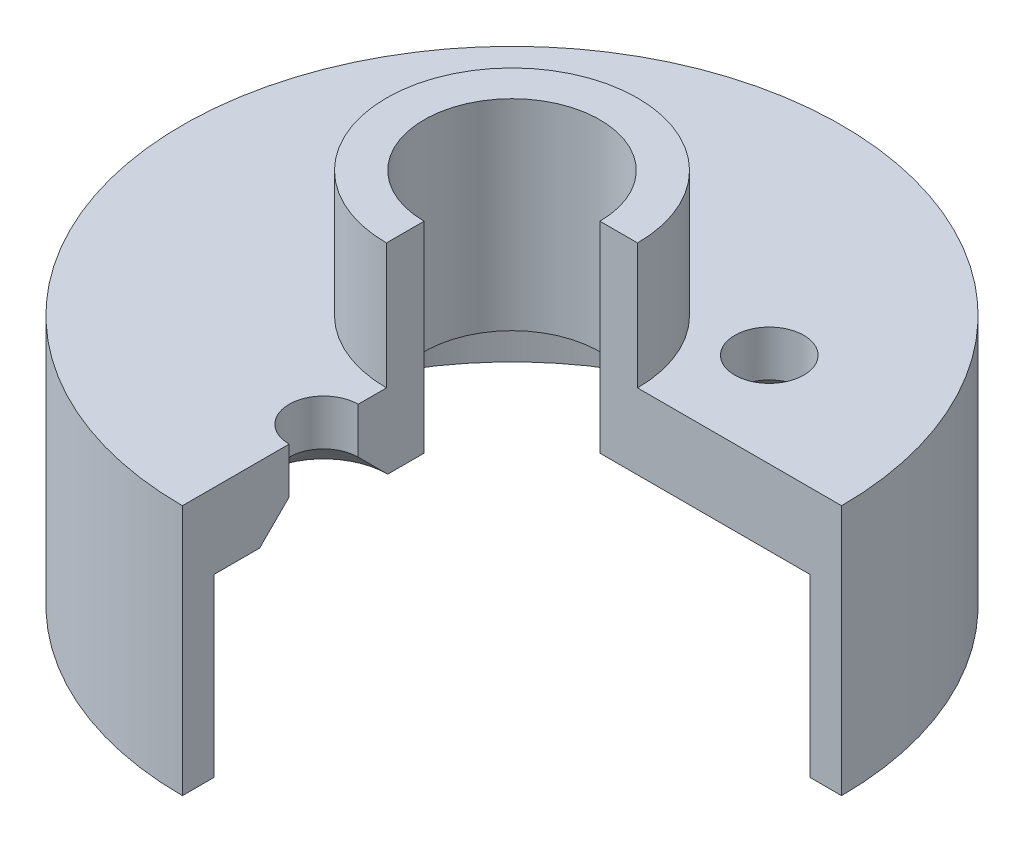
ISO-10303-21;
HEADER;
FILE_DESCRIPTION(('STEP AP214'),'2;1');
FILE_NAME('part.step','',(''),(''),'','','');
FILE_SCHEMA(('AUTOMOTIVE_DESIGN { 1 0 10303 214 1 1 1 1 }'));
ENDSEC;
DATA;
#1=APPLICATION_CONTEXT('core data for automotive mechanical design processes');
#2=APPLICATION_PROTOCOL_DEFINITION('international standard','automotive_design',2000,#1);
#3=PRODUCT_CONTEXT('',#1,'mechanical');
#4=PRODUCT('Part','Part','',(#3));
#5=PRODUCT_RELATED_PRODUCT_CATEGORY('part','',(#4));
#6=PRODUCT_DEFINITION_FORMATION('','',#4);
#7=PRODUCT_DEFINITION_CONTEXT('part definition',#1,'design');
#8=PRODUCT_DEFINITION('design','',#6,#7);
#9=PRODUCT_DEFINITION_SHAPE('','',#8);
#10=(LENGTH_UNIT() NAMED_UNIT(*) SI_UNIT(.MILLI.,.METRE.));
#11=(NAMED_UNIT(*) PLANE_ANGLE_UNIT() SI_UNIT($,.RADIAN.));
#12=(NAMED_UNIT(*) SI_UNIT($,.STERADIAN.) SOLID_ANGLE_UNIT());
#13=UNCERTAINTY_MEASURE_WITH_UNIT(LENGTH_MEASURE(1.E-05),#10,'distance_accuracy_value','');
#14=(GEOMETRIC_REPRESENTATION_CONTEXT(3) GLOBAL_UNCERTAINTY_ASSIGNED_CONTEXT((#13)) GLOBAL_UNIT_ASSIGNED_CONTEXT((#10,
#11,#12)) REPRESENTATION_CONTEXT('',''));
#15=CARTESIAN_POINT('',(0.,0.,0.));
#16=DIRECTION('',(0.,0.,1.));
#17=DIRECTION('',(1.,0.,0.));
#18=AXIS2_PLACEMENT_3D('',#15,#16,#17);
#19=CARTESIAN_POINT('',(0.,30.3936773445756,-20.));
#20=DIRECTION('',(0.,1.,0.));
#21=DIRECTION('',(0.,0.,1.));
#22=AXIS2_PLACEMENT_3D('',#19,#20,#21);
#23=PLANE('',#22);
#24=DIRECTION('',(1.,0.,0.));
#25=VECTOR('',#24,1.);
#26=CARTESIAN_POINT('',(0.,30.3936773445756,0.));
#27=LINE('',#26,#25);
#28=CARTESIAN_POINT('',(14.,30.3936773445756,0.));
#29=VERTEX_POINT('',#28);
#30=CARTESIAN_POINT('',(20.,30.3936773445756,0.));
#31=VERTEX_POINT('',#30);
#32=EDGE_CURVE('E215',#29,#31,#27,.T.);
#33=ORIENTED_EDGE('',*,*,#32,.T.);
#34=CARTESIAN_POINT('',(0.,30.3936773445756,0.));
#35=DIRECTION('',(0.,-1.,0.));
#36=DIRECTION('',(0.,0.,-1.));
#37=AXIS2_PLACEMENT_3D('',#34,#35,#36);
#38=CIRCLE('',#37,20.);
#39=CARTESIAN_POINT('',(0.,30.3936773445756,20.));
#40=VERTEX_POINT('',#39);
#41=EDGE_CURVE('E164',#40,#31,#38,.T.);
#42=ORIENTED_EDGE('',*,*,#41,.F.);
#43=DIRECTION('',(0.,0.,-1.));
#44=VECTOR('',#43,1.);
#45=CARTESIAN_POINT('',(0.,30.3936773445756,66.3150525087515));
#46=LINE('',#45,#44);
#47=CARTESIAN_POINT('',(0.,30.3936773445756,14.));
#48=VERTEX_POINT('',#47);
#49=EDGE_CURVE('E220',#40,#48,#46,.T.);
#50=ORIENTED_EDGE('',*,*,#49,.T.);
#51=CARTESIAN_POINT('',(0.,30.3936773445756,0.));
#52=DIRECTION('',(0.,-1.,0.));
#53=DIRECTION('',(0.,0.,-1.));
#54=AXIS2_PLACEMENT_3D('',#51,#52,#53);
#55=CIRCLE('',#54,14.);
#56=EDGE_CURVE('E158',#48,#29,#55,.T.);
#57=ORIENTED_EDGE('',*,*,#56,.T.);
#58=EDGE_LOOP('',(#33,#42,#50,#57));
#59=FACE_BOUND('',#58,.T.);
#60=ADVANCED_FACE('F41',(#59),#23,.T.);
#61=CARTESIAN_POINT('',(0.,0.,0.));
#62=DIRECTION('',(0.,-1.,0.));
#63=DIRECTION('',(0.,0.,-1.));
#64=AXIS2_PLACEMENT_3D('',#61,#62,#63);
#65=CYLINDRICAL_SURFACE('',#64,14.);
#66=DIRECTION('',(0.,-1.,0.));
#67=VECTOR('',#66,1.);
#68=CARTESIAN_POINT('',(14.,0.,0.));
#69=LINE('',#68,#67);
#70=CARTESIAN_POINT('',(14.,-1.60632265542437,0.));
#71=VERTEX_POINT('',#70);
#72=EDGE_CURVE('E236',#29,#71,#69,.T.);
#73=ORIENTED_EDGE('',*,*,#72,.F.);
#74=ORIENTED_EDGE('',*,*,#56,.F.);
#75=DIRECTION('',(0.,-1.,0.));
#76=VECTOR('',#75,1.);
#77=CARTESIAN_POINT('',(0.,0.,14.));
#78=LINE('',#77,#76);
#79=CARTESIAN_POINT('',(0.,-1.60632265542437,14.));
#80=VERTEX_POINT('',#79);
#81=EDGE_CURVE('E228',#80,#48,#78,.F.);
#82=ORIENTED_EDGE('',*,*,#81,.F.);
#83=CARTESIAN_POINT('',(0.,-1.60632265542437,0.));
#84=DIRECTION('',(0.,-1.,0.));
#85=DIRECTION('',(0.,0.,-1.));
#86=AXIS2_PLACEMENT_3D('',#83,#84,#85);
#87=CIRCLE('',#86,14.);
#88=EDGE_CURVE('E154',#80,#71,#87,.T.);
#89=ORIENTED_EDGE('',*,*,#88,.T.);
#90=EDGE_LOOP('',(#73,#74,#82,#89));
#91=FACE_BOUND('',#90,.T.);
#92=ADVANCED_FACE('F261',(#91),#65,.F.);
#93=CARTESIAN_POINT('',(0.,-1.60632265542437,-14.));
#94=DIRECTION('',(0.,-1.,0.));
#95=DIRECTION('',(0.,0.,-1.));
#96=AXIS2_PLACEMENT_3D('',#93,#94,#95);
#97=PLANE('',#96);
#98=DIRECTION('',(1.,0.,0.));
#99=VECTOR('',#98,1.);
#100=CARTESIAN_POINT('',(0.,-1.60632265542437,0.));
#101=LINE('',#100,#99);
#102=CARTESIAN_POINT('',(47.5,-1.60632265542437,0.));
#103=VERTEX_POINT('',#102);
#104=EDGE_CURVE('E237',#71,#103,#101,.T.);
#105=ORIENTED_EDGE('',*,*,#104,.F.);
#106=ORIENTED_EDGE('',*,*,#88,.F.);
#107=DIRECTION('',(0.,0.,-1.));
#108=VECTOR('',#107,1.);
#109=CARTESIAN_POINT('',(0.,-1.60632265542437,-14.));
#110=LINE('',#109,#108);
#111=CARTESIAN_POINT('',(0.,-1.60632265542437,19.8));
#112=VERTEX_POINT('',#111);
#113=EDGE_CURVE('E226',#112,#80,#110,.T.);
#114=ORIENTED_EDGE('',*,*,#113,.F.);
#115=CARTESIAN_POINT('',(0.,-1.60632265542437,30.));
#116=DIRECTION('',(0.,-1.,0.));
#117=DIRECTION('',(0.,0.,-1.));
#118=AXIS2_PLACEMENT_3D('',#115,#116,#117);
#119=CIRCLE('',#118,10.2);
#120=CARTESIAN_POINT('',(0.,-1.60632265542437,40.2));
#121=VERTEX_POINT('',#120);
#122=EDGE_CURVE('E168',#121,#112,#119,.T.);
#123=ORIENTED_EDGE('',*,*,#122,.F.);
#124=CARTESIAN_POINT('',(0.,-1.60632265542437,47.5));
#125=VERTEX_POINT('',#124);
#126=EDGE_CURVE('E62',#125,#121,#110,.T.);
#127=ORIENTED_EDGE('',*,*,#126,.F.);
#128=CARTESIAN_POINT('',(0.,-1.60632265542437,0.));
#129=DIRECTION('',(0.,-1.,0.));
#130=DIRECTION('',(0.,0.,-1.));
#131=AXIS2_PLACEMENT_3D('',#128,#129,#130);
#132=CIRCLE('',#131,47.5);
#133=EDGE_CURVE('E150',#125,#103,#132,.T.);
#134=ORIENTED_EDGE('',*,*,#133,.T.);
#135=EDGE_LOOP('',(#105,#106,#114,#123,#127,#134));
#136=FACE_BOUND('',#135,.T.);
#137=CARTESIAN_POINT('',(25.9807621135333,-1.60632265542437,-14.9999999999998));
#138=DIRECTION('',(0.,-1.,0.));
#139=DIRECTION('',(0.,0.,-1.));
#140=AXIS2_PLACEMENT_3D('',#137,#138,#139);
#141=CIRCLE('',#140,10.2);
#142=CARTESIAN_POINT('',(25.9807621135333,-1.60632265542437,-25.1999999999998));
#143=VERTEX_POINT('',#142);
#144=EDGE_CURVE('E238',#143,#143,#141,.T.);
#145=ORIENTED_EDGE('',*,*,#144,.F.);
#146=EDGE_LOOP('',(#145));
#147=FACE_BOUND('',#146,.T.);
#148=CARTESIAN_POINT('',(-25.9807621135331,-1.60632265542437,-15.0000000000001));
#149=DIRECTION('',(0.,-1.,0.));
#150=DIRECTION('',(0.,0.,-1.));
#151=AXIS2_PLACEMENT_3D('',#148,#149,#150);
#152=CIRCLE('',#151,10.2);
#153=CARTESIAN_POINT('',(-25.9807621135331,-1.60632265542437,-25.2000000000001));
#154=VERTEX_POINT('',#153);
#155=EDGE_CURVE('E175',#154,#154,#152,.T.);
#156=ORIENTED_EDGE('',*,*,#155,.F.);
#157=EDGE_LOOP('',(#156));
#158=FACE_BOUND('',#157,.T.);
#159=ADVANCED_FACE('F256',(#136,#147,#158),#97,.T.);
#160=CARTESIAN_POINT('',(0.,0.,0.));
#161=DIRECTION('',(0.,-1.,0.));
#162=DIRECTION('',(0.,0.,-1.));
#163=AXIS2_PLACEMENT_3D('',#160,#161,#162);
#164=CYLINDRICAL_SURFACE('',#163,47.5);
#165=DIRECTION('',(0.,-1.,0.));
#166=VECTOR('',#165,1.);
#167=CARTESIAN_POINT('',(47.5,0.,0.));
#168=LINE('',#167,#166);
#169=CARTESIAN_POINT('',(47.5,-29.6063226554244,0.));
#170=VERTEX_POINT('',#169);
#171=EDGE_CURVE('E232',#103,#170,#168,.T.);
#172=ORIENTED_EDGE('',*,*,#171,.F.);
#173=ORIENTED_EDGE('',*,*,#133,.F.);
#174=DIRECTION('',(0.,-1.,0.));
#175=VECTOR('',#174,1.);
#176=CARTESIAN_POINT('',(0.,0.,47.5));
#177=LINE('',#176,#175);
#178=CARTESIAN_POINT('',(0.,-29.6063226554244,47.5));
#179=VERTEX_POINT('',#178);
#180=EDGE_CURVE('E223',#179,#125,#177,.F.);
#181=ORIENTED_EDGE('',*,*,#180,.F.);
#182=CARTESIAN_POINT('',(0.,-29.6063226554244,0.));
#183=DIRECTION('',(0.,-1.,0.));
#184=DIRECTION('',(0.,0.,-1.));
#185=AXIS2_PLACEMENT_3D('',#182,#183,#184);
#186=CIRCLE('',#185,47.5);
#187=EDGE_CURVE('E137',#179,#170,#186,.T.);
#188=ORIENTED_EDGE('',*,*,#187,.T.);
#189=EDGE_LOOP('',(#172,#173,#181,#188));
#190=FACE_BOUND('',#189,.T.);
#191=ADVANCED_FACE('F257',(#190),#164,.F.);
#192=CARTESIAN_POINT('',(0.,-29.6063226554244,-47.5));
#193=DIRECTION('',(0.,-1.,0.));
#194=DIRECTION('',(0.,0.,-1.));
#195=AXIS2_PLACEMENT_3D('',#192,#193,#194);
#196=PLANE('',#195);
#197=DIRECTION('',(1.,0.,0.));
#198=VECTOR('',#197,1.);
#199=CARTESIAN_POINT('',(0.,-29.6063226554244,0.));
#200=LINE('',#199,#198);
#201=CARTESIAN_POINT('',(52.5,-29.6063226554244,0.));
#202=VERTEX_POINT('',#201);
#203=EDGE_CURVE('E139',#170,#202,#200,.T.);
#204=ORIENTED_EDGE('',*,*,#203,.F.);
#205=ORIENTED_EDGE('',*,*,#187,.F.);
#206=DIRECTION('',(0.,0.,-1.));
#207=VECTOR('',#206,1.);
#208=CARTESIAN_POINT('',(0.,-29.6063226554244,66.3150525087515));
#209=LINE('',#208,#207);
#210=CARTESIAN_POINT('',(0.,-29.6063226554244,52.5));
#211=VERTEX_POINT('',#210);
#212=EDGE_CURVE('E121',#211,#179,#209,.T.);
#213=ORIENTED_EDGE('',*,*,#212,.F.);
#214=CARTESIAN_POINT('',(0.,-29.6063226554244,0.));
#215=DIRECTION('',(0.,-1.,0.));
#216=DIRECTION('',(0.,0.,-1.));
#217=AXIS2_PLACEMENT_3D('',#214,#215,#216);
#218=CIRCLE('',#217,52.5);
#219=EDGE_CURVE('E140',#211,#202,#218,.T.);
#220=ORIENTED_EDGE('',*,*,#219,.T.);
#221=EDGE_LOOP('',(#204,#205,#213,#220));
#222=FACE_BOUND('',#221,.T.);
#223=ADVANCED_FACE('F138',(#222),#196,.T.);
#224=CARTESIAN_POINT('',(0.,0.,0.));
#225=DIRECTION('',(0.,-1.,0.));
#226=DIRECTION('',(0.,0.,-1.));
#227=AXIS2_PLACEMENT_3D('',#224,#225,#226);
#228=CYLINDRICAL_SURFACE('',#227,52.5);
#229=DIRECTION('',(0.,-1.,0.));
#230=VECTOR('',#229,1.);
#231=CARTESIAN_POINT('',(52.5,0.,0.));
#232=LINE('',#231,#230);
#233=CARTESIAN_POINT('',(52.5,10.3936773445756,0.));
#234=VERTEX_POINT('',#233);
#235=EDGE_CURVE('E145',#202,#234,#232,.F.);
#236=ORIENTED_EDGE('',*,*,#235,.F.);
#237=ORIENTED_EDGE('',*,*,#219,.F.);
#238=DIRECTION('',(0.,-1.,0.));
#239=VECTOR('',#238,1.);
#240=CARTESIAN_POINT('',(0.,0.,52.5));
#241=LINE('',#240,#239);
#242=CARTESIAN_POINT('',(0.,10.3936773445756,52.5));
#243=VERTEX_POINT('',#242);
#244=EDGE_CURVE('E120',#243,#211,#241,.T.);
#245=ORIENTED_EDGE('',*,*,#244,.F.);
#246=CARTESIAN_POINT('',(0.,10.3936773445756,0.));
#247=DIRECTION('',(0.,-1.,0.));
#248=DIRECTION('',(0.,0.,-1.));
#249=AXIS2_PLACEMENT_3D('',#246,#247,#248);
#250=CIRCLE('',#249,52.5);
#251=EDGE_CURVE('E144',#243,#234,#250,.T.);
#252=ORIENTED_EDGE('',*,*,#251,.T.);
#253=EDGE_LOOP('',(#236,#237,#245,#252));
#254=FACE_BOUND('',#253,.T.);
#255=ADVANCED_FACE('F141',(#254),#228,.T.);
#256=CARTESIAN_POINT('',(0.,10.3936773445756,-52.5));
#257=DIRECTION('',(0.,1.,0.));
#258=DIRECTION('',(0.,0.,1.));
#259=AXIS2_PLACEMENT_3D('',#256,#257,#258);
#260=PLANE('',#259);
#261=DIRECTION('',(-1.,0.,0.));
#262=VECTOR('',#261,1.);
#263=CARTESIAN_POINT('',(0.,10.3936773445756,0.));
#264=LINE('',#263,#262);
#265=CARTESIAN_POINT('',(20.,10.3936773445756,0.));
#266=VERTEX_POINT('',#265);
#267=EDGE_CURVE('E53',#234,#266,#264,.T.);
#268=ORIENTED_EDGE('',*,*,#267,.F.);
#269=ORIENTED_EDGE('',*,*,#251,.F.);
#270=DIRECTION('',(0.,0.,1.));
#271=VECTOR('',#270,1.);
#272=CARTESIAN_POINT('',(0.,10.3936773445756,-52.5));
#273=LINE('',#272,#271);
#274=CARTESIAN_POINT('',(0.,10.3936773445756,35.5));
#275=VERTEX_POINT('',#274);
#276=EDGE_CURVE('E127',#275,#243,#273,.T.);
#277=ORIENTED_EDGE('',*,*,#276,.F.);
#278=CARTESIAN_POINT('',(0.,10.3936773445756,30.));
#279=DIRECTION('',(0.,1.,0.));
#280=DIRECTION('',(0.,0.,1.));
#281=AXIS2_PLACEMENT_3D('',#278,#279,#280);
#282=CIRCLE('',#281,5.5);
#283=CARTESIAN_POINT('',(0.,10.3936773445756,24.5));
#284=VERTEX_POINT('',#283);
#285=EDGE_CURVE('E165',#284,#275,#282,.T.);
#286=ORIENTED_EDGE('',*,*,#285,.F.);
#287=CARTESIAN_POINT('',(0.,10.3936773445756,20.));
#288=VERTEX_POINT('',#287);
#289=EDGE_CURVE('E204',#288,#284,#273,.T.);
#290=ORIENTED_EDGE('',*,*,#289,.F.);
#291=CARTESIAN_POINT('',(0.,10.3936773445756,0.));
#292=DIRECTION('',(0.,-1.,0.));
#293=DIRECTION('',(0.,0.,-1.));
#294=AXIS2_PLACEMENT_3D('',#291,#292,#293);
#295=CIRCLE('',#294,20.);
#296=EDGE_CURVE('E149',#288,#266,#295,.T.);
#297=ORIENTED_EDGE('',*,*,#296,.T.);
#298=EDGE_LOOP('',(#268,#269,#277,#286,#290,#297));
#299=FACE_BOUND('',#298,.T.);
#300=CARTESIAN_POINT('',(25.9807621135333,10.3936773445756,-14.9999999999998));
#301=DIRECTION('',(0.,1.,0.));
#302=DIRECTION('',(0.,0.,1.));
#303=AXIS2_PLACEMENT_3D('',#300,#301,#302);
#304=CIRCLE('',#303,5.5);
#305=CARTESIAN_POINT('',(25.9807621135333,10.3936773445756,-9.49999999999976));
#306=VERTEX_POINT('',#305);
#307=EDGE_CURVE('E172',#306,#306,#304,.T.);
#308=ORIENTED_EDGE('',*,*,#307,.F.);
#309=EDGE_LOOP('',(#308));
#310=FACE_BOUND('',#309,.T.);
#311=CARTESIAN_POINT('',(-25.9807621135331,10.3936773445756,-15.0000000000001));
#312=DIRECTION('',(0.,1.,0.));
#313=DIRECTION('',(0.,0.,1.));
#314=AXIS2_PLACEMENT_3D('',#311,#312,#313);
#315=CIRCLE('',#314,5.5);
#316=CARTESIAN_POINT('',(-25.9807621135331,10.3936773445756,-9.50000000000012));
#317=VERTEX_POINT('',#316);
#318=EDGE_CURVE('E170',#317,#317,#315,.T.);
#319=ORIENTED_EDGE('',*,*,#318,.F.);
#320=EDGE_LOOP('',(#319));
#321=FACE_BOUND('',#320,.T.);
#322=ADVANCED_FACE('F205',(#299,#310,#321),#260,.T.);
#323=CARTESIAN_POINT('',(0.,0.,0.));
#324=DIRECTION('',(0.,-1.,0.));
#325=DIRECTION('',(0.,0.,-1.));
#326=AXIS2_PLACEMENT_3D('',#323,#324,#325);
#327=CYLINDRICAL_SURFACE('',#326,20.);
#328=DIRECTION('',(0.,-1.,0.));
#329=VECTOR('',#328,1.);
#330=CARTESIAN_POINT('',(20.,0.,0.));
#331=LINE('',#330,#329);
#332=EDGE_CURVE('E11',#266,#31,#331,.F.);
#333=ORIENTED_EDGE('',*,*,#332,.F.);
#334=ORIENTED_EDGE('',*,*,#296,.F.);
#335=DIRECTION('',(0.,-1.,0.));
#336=VECTOR('',#335,1.);
#337=CARTESIAN_POINT('',(0.,0.,20.));
#338=LINE('',#337,#336);
#339=EDGE_CURVE('E208',#40,#288,#338,.T.);
#340=ORIENTED_EDGE('',*,*,#339,.F.);
#341=ORIENTED_EDGE('',*,*,#41,.T.);
#342=EDGE_LOOP('',(#333,#334,#340,#341));
#343=FACE_BOUND('',#342,.T.);
#344=ADVANCED_FACE('F210',(#343),#327,.T.);
#345=CARTESIAN_POINT('',(0.,-1.60632265542437,30.));
#346=DIRECTION('',(0.,-1.,0.));
#347=DIRECTION('',(0.,0.,-1.));
#348=AXIS2_PLACEMENT_3D('',#345,#346,#347);
#349=CYLINDRICAL_SURFACE('',#348,5.5);
#350=CARTESIAN_POINT('',(0.,3.09367734457563,30.));
#351=DIRECTION('',(0.,-1.,0.));
#352=DIRECTION('',(0.,0.,-1.));
#353=AXIS2_PLACEMENT_3D('',#350,#351,#352);
#354=CIRCLE('',#353,5.5);
#355=CARTESIAN_POINT('',(0.,3.09367734457563,35.5));
#356=VERTEX_POINT('',#355);
#357=CARTESIAN_POINT('',(0.,3.09367734457563,24.5));
#358=VERTEX_POINT('',#357);
#359=EDGE_CURVE('E167',#356,#358,#354,.T.);
#360=ORIENTED_EDGE('',*,*,#359,.T.);
#361=DIRECTION('',(0.,-1.,0.));
#362=VECTOR('',#361,1.);
#363=CARTESIAN_POINT('',(0.,-1.60632265542437,24.5));
#364=LINE('',#363,#362);
#365=EDGE_CURVE('E190',#358,#284,#364,.F.);
#366=ORIENTED_EDGE('',*,*,#365,.T.);
#367=ORIENTED_EDGE('',*,*,#285,.T.);
#368=DIRECTION('',(0.,-1.,0.));
#369=VECTOR('',#368,1.);
#370=CARTESIAN_POINT('',(0.,-1.60632265542437,35.5));
#371=LINE('',#370,#369);
#372=EDGE_CURVE('E195',#275,#356,#371,.T.);
#373=ORIENTED_EDGE('',*,*,#372,.T.);
#374=EDGE_LOOP('',(#360,#366,#367,#373));
#375=FACE_BOUND('',#374,.T.);
#376=ADVANCED_FACE('F188',(#375),#349,.F.);
#377=CARTESIAN_POINT('',(0.,-1.60632265542437,30.));
#378=DIRECTION('',(0.,-1.,0.));
#379=DIRECTION('',(0.,0.,-1.));
#380=AXIS2_PLACEMENT_3D('',#377,#378,#379);
#381=CONICAL_SURFACE('',#380,10.2,0.785398163397449);
#382=ORIENTED_EDGE('',*,*,#122,.T.);
#383=DIRECTION('',(0.,-0.707106781186547,-0.707106781186548));
#384=VECTOR('',#383,1.);
#385=CARTESIAN_POINT('',(0.,8.59367734457562,30.));
#386=LINE('',#385,#384);
#387=EDGE_CURVE('E48',#112,#358,#386,.F.);
#388=ORIENTED_EDGE('',*,*,#387,.T.);
#389=ORIENTED_EDGE('',*,*,#359,.F.);
#390=DIRECTION('',(0.,0.707106781186547,-0.707106781186548));
#391=VECTOR('',#390,1.);
#392=CARTESIAN_POINT('',(0.,8.59367734457562,30.));
#393=LINE('',#392,#391);
#394=EDGE_CURVE('E161',#356,#121,#393,.F.);
#395=ORIENTED_EDGE('',*,*,#394,.T.);
#396=EDGE_LOOP('',(#382,#388,#389,#395));
#397=FACE_BOUND('',#396,.T.);
#398=ADVANCED_FACE('F185',(#397),#381,.F.);
#399=CARTESIAN_POINT('',(-25.9807621135331,-1.60632265542437,-15.0000000000001));
#400=DIRECTION('',(0.,-1.,0.));
#401=DIRECTION('',(0.,0.,-1.));
#402=AXIS2_PLACEMENT_3D('',#399,#400,#401);
#403=CYLINDRICAL_SURFACE('',#402,5.5);
#404=ORIENTED_EDGE('',*,*,#318,.T.);
#405=EDGE_LOOP('',(#404));
#406=FACE_BOUND('',#405,.T.);
#407=CARTESIAN_POINT('',(-25.9807621135331,3.09367734457563,-15.0000000000001));
#408=DIRECTION('',(0.,-1.,0.));
#409=DIRECTION('',(0.,0.,-1.));
#410=AXIS2_PLACEMENT_3D('',#407,#408,#409);
#411=CIRCLE('',#410,5.5);
#412=CARTESIAN_POINT('',(-25.9807621135331,3.09367734457563,-20.5000000000001));
#413=VERTEX_POINT('',#412);
#414=EDGE_CURVE('E171',#413,#413,#411,.T.);
#415=ORIENTED_EDGE('',*,*,#414,.T.);
#416=EDGE_LOOP('',(#415));
#417=FACE_BOUND('',#416,.T.);
#418=ADVANCED_FACE('F247',(#406,#417),#403,.F.);
#419=CARTESIAN_POINT('',(-25.9807621135331,-1.60632265542437,-15.0000000000001));
#420=DIRECTION('',(0.,-1.,0.));
#421=DIRECTION('',(0.,0.,-1.));
#422=AXIS2_PLACEMENT_3D('',#419,#420,#421);
#423=CONICAL_SURFACE('',#422,10.2,0.785398163397448);
#424=ORIENTED_EDGE('',*,*,#414,.F.);
#425=EDGE_LOOP('',(#424));
#426=FACE_BOUND('',#425,.T.);
#427=ORIENTED_EDGE('',*,*,#155,.T.);
#428=EDGE_LOOP('',(#427));
#429=FACE_BOUND('',#428,.T.);
#430=ADVANCED_FACE('F253',(#426,#429),#423,.F.);
#431=CARTESIAN_POINT('',(25.9807621135333,-1.60632265542437,-14.9999999999998));
#432=DIRECTION('',(0.,-1.,0.));
#433=DIRECTION('',(0.,0.,-1.));
#434=AXIS2_PLACEMENT_3D('',#431,#432,#433);
#435=CYLINDRICAL_SURFACE('',#434,5.5);
#436=ORIENTED_EDGE('',*,*,#307,.T.);
#437=EDGE_LOOP('',(#436));
#438=FACE_BOUND('',#437,.T.);
#439=CARTESIAN_POINT('',(25.9807621135333,3.09367734457563,-14.9999999999998));
#440=DIRECTION('',(0.,-1.,0.));
#441=DIRECTION('',(0.,0.,-1.));
#442=AXIS2_PLACEMENT_3D('',#439,#440,#441);
#443=CIRCLE('',#442,5.5);
#444=CARTESIAN_POINT('',(25.9807621135333,3.09367734457563,-20.4999999999998));
#445=VERTEX_POINT('',#444);
#446=EDGE_CURVE('E178',#445,#445,#443,.T.);
#447=ORIENTED_EDGE('',*,*,#446,.T.);
#448=EDGE_LOOP('',(#447));
#449=FACE_BOUND('',#448,.T.);
#450=ADVANCED_FACE('F255',(#438,#449),#435,.F.);
#451=CARTESIAN_POINT('',(25.9807621135333,-1.60632265542437,-14.9999999999998));
#452=DIRECTION('',(0.,-1.,0.));
#453=DIRECTION('',(0.,0.,-1.));
#454=AXIS2_PLACEMENT_3D('',#451,#452,#453);
#455=CONICAL_SURFACE('',#454,10.2,0.785398163397449);
#456=ORIENTED_EDGE('',*,*,#446,.F.);
#457=EDGE_LOOP('',(#456));
#458=FACE_BOUND('',#457,.T.);
#459=ORIENTED_EDGE('',*,*,#144,.T.);
#460=EDGE_LOOP('',(#459));
#461=FACE_BOUND('',#460,.T.);
#462=ADVANCED_FACE('F281',(#458,#461),#455,.F.);
#463=CARTESIAN_POINT('',(0.,30.3936773445756,66.3150525087515));
#464=DIRECTION('',(-1.,0.,0.));
#465=DIRECTION('',(0.,0.,1.));
#466=AXIS2_PLACEMENT_3D('',#463,#464,#465);
#467=PLANE('',#466);
#468=ORIENTED_EDGE('',*,*,#180,.T.);
#469=ORIENTED_EDGE('',*,*,#126,.T.);
#470=ORIENTED_EDGE('',*,*,#394,.F.);
#471=ORIENTED_EDGE('',*,*,#372,.F.);
#472=ORIENTED_EDGE('',*,*,#276,.T.);
#473=ORIENTED_EDGE('',*,*,#244,.T.);
#474=ORIENTED_EDGE('',*,*,#212,.T.);
#475=EDGE_LOOP('',(#468,#469,#470,#471,#472,#473,#474));
#476=FACE_BOUND('',#475,.T.);
#477=ADVANCED_FACE('F125',(#476),#467,.F.);
#478=ORIENTED_EDGE('',*,*,#339,.T.);
#479=ORIENTED_EDGE('',*,*,#289,.T.);
#480=ORIENTED_EDGE('',*,*,#365,.F.);
#481=ORIENTED_EDGE('',*,*,#387,.F.);
#482=ORIENTED_EDGE('',*,*,#113,.T.);
#483=ORIENTED_EDGE('',*,*,#81,.T.);
#484=ORIENTED_EDGE('',*,*,#49,.F.);
#485=EDGE_LOOP('',(#478,#479,#480,#481,#482,#483,#484));
#486=FACE_BOUND('',#485,.T.);
#487=ADVANCED_FACE('F382',(#486),#467,.F.);
#488=CARTESIAN_POINT('',(0.,30.3936773445756,0.));
#489=DIRECTION('',(0.,0.,-1.));
#490=DIRECTION('',(-1.,0.,0.));
#491=AXIS2_PLACEMENT_3D('',#488,#489,#490);
#492=PLANE('',#491);
#493=ORIENTED_EDGE('',*,*,#72,.T.);
#494=ORIENTED_EDGE('',*,*,#104,.T.);
#495=ORIENTED_EDGE('',*,*,#171,.T.);
#496=ORIENTED_EDGE('',*,*,#203,.T.);
#497=ORIENTED_EDGE('',*,*,#235,.T.);
#498=ORIENTED_EDGE('',*,*,#267,.T.);
#499=ORIENTED_EDGE('',*,*,#332,.T.);
#500=ORIENTED_EDGE('',*,*,#32,.F.);
#501=EDGE_LOOP('',(#493,#494,#495,#496,#497,#498,#499,#500));
#502=FACE_BOUND('',#501,.T.);
#503=ADVANCED_FACE('F211',(#502),#492,.F.);
#504=CLOSED_SHELL('',(#60,#92,#159,#191,#223,#255,#322,#344,#376,#398,#418,#430,#450,#462,#477,
#487,#503));
#505=MANIFOLD_SOLID_BREP('B2',#504);
#506=ADVANCED_BREP_SHAPE_REPRESENTATION('',(#18,#505),#14);
#507=SHAPE_DEFINITION_REPRESENTATION(#9,#506);
ENDSEC;
END-ISO-10303-21;
